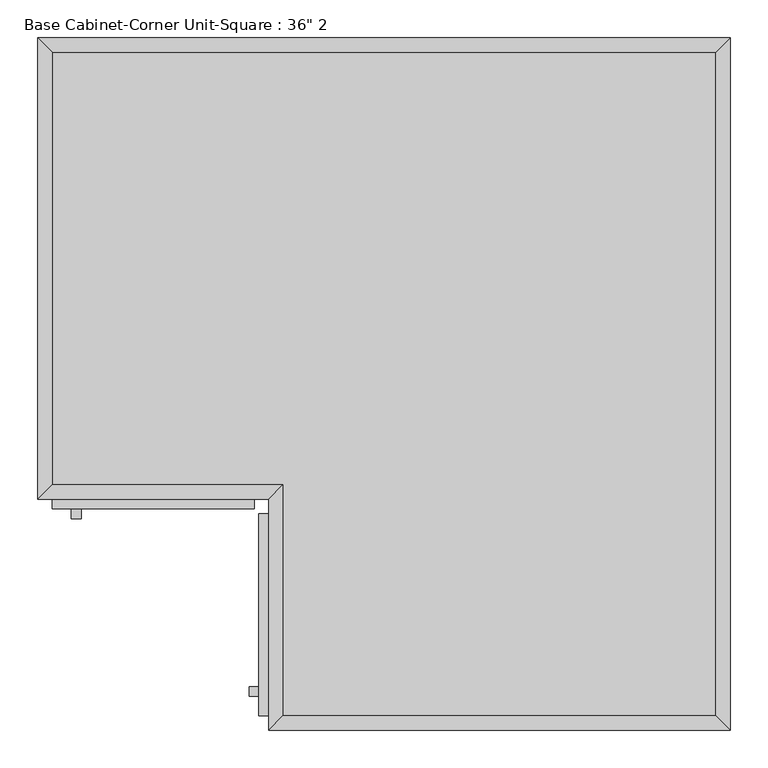
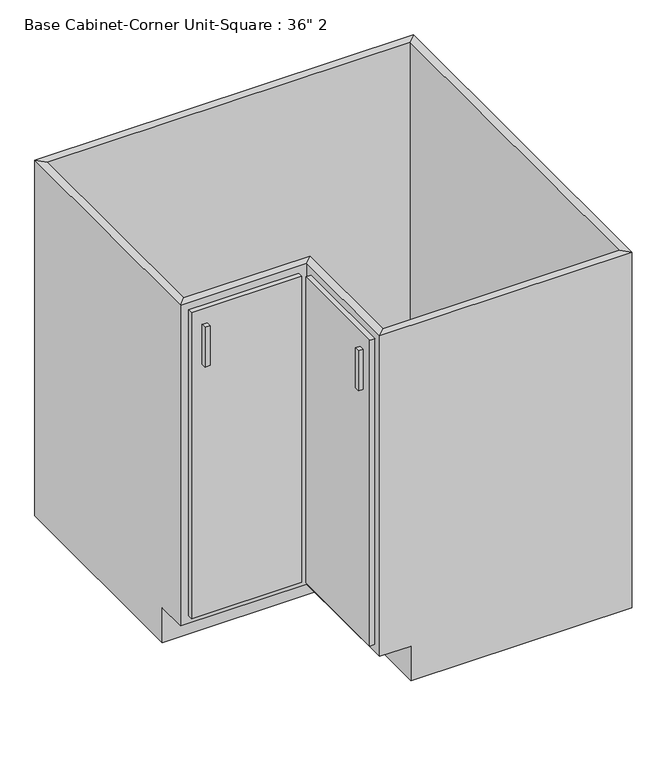
"""IFC4 building model written with IfcOpenShell, lengths in millimetres: furniture geometry."""

from ifc_helpers import new_model, si_unit, frame, origin, place, context, project, spatial, polyline, outline, extrude, faceted_brep, source, transform, mapped, element, save


def furniture_13b99e4d(model_context):
    return source(origin(), model_context, "Body", "SolidModel", [
        extrude(outline(polyline([(507.6877049, -19.05), (507.6877049, -895.35), (-63.8122951, -895.35), (-63.8122951, -590.55), (-368.6122951, -590.55), (-368.6122951, -19.05), (507.6877049, -19.05)])), frame((0.0, 0.0, 88.9), z_axis=(0.0, 0.0, 1.0), x_axis=(1.0, 0.0, 0.0)), (0.0, 0.0, 1.0), 19.05),
        extrude(outline(polyline([(-101.9122951, -622.3), (-368.6122951, -622.3), (-368.6122951, -609.6), (-101.9122951, -609.6), (-101.9122951, -622.3)])), frame((0.0, 0.0, 107.95), z_axis=(0.0, 0.0, 1.0), x_axis=(1.0, 0.0, 0.0)), (0.0, 0.0, 1.0), 781.05),
        extrude(outline(polyline([(-330.5122951, -635.0), (-343.2122951, -635.0), (-343.2122951, -622.3), (-330.5122951, -622.3), (-330.5122951, -635.0)])), frame((0.0, 0.0, 749.3), z_axis=(0.0, 0.0, 1.0), x_axis=(1.0, 0.0, 0.0)), (0.0, 0.0, 1.0), 101.6),
        extrude(outline(polyline([(-82.8622951, -628.65), (-82.8622951, -895.35), (-95.5622951, -895.35), (-95.5622951, -628.65), (-82.8622951, -628.65)])), frame((0.0, 0.0, 107.95), z_axis=(0.0, 0.0, 1.0), x_axis=(1.0, 0.0, 0.0)), (0.0, 0.0, 1.0), 781.05),
        extrude(outline(polyline([(-95.5622951, -857.25), (-95.5622951, -869.95), (-108.2622951, -869.95), (-108.2622951, -857.25), (-95.5622951, -857.25)])), frame((0.0, 0.0, 749.3), z_axis=(0.0, 0.0, 1.0), x_axis=(1.0, 0.0, 0.0)), (0.0, 0.0, 1.0), 101.6),
        faceted_brep([(-368.6122951, -533.4, 88.9), (-6.6622951, -533.4, 88.9), (-6.6622951, -895.35, 88.9), (507.6877049, -895.35, 88.9), (507.6877049, -19.05, 88.9), (-368.6122951, -19.05, 88.9), (526.7377049, 0.0, 0.0), (526.7377049, -914.4, 0.0), (-6.6622951, -914.4, 0.0), (-6.6622951, -533.4, 0.0), (-387.6622951, -533.4, 0.0), (-387.6622951, 0.0, 0.0), (-387.6622951, 0.0, 908.05), (526.7377049, 0.0, 908.05), (-387.6622951, -533.4, 88.9), (-387.6622951, -609.6, 88.9), (-387.6622951, -609.6, 908.05), (-6.6622951, -914.4, 88.9), (526.7377049, -914.4, 908.05), (-82.8622951, -914.4, 908.05), (-82.8622951, -914.4, 88.9), (507.6877049, -895.35, 908.05), (-63.8122951, -895.35, 88.9), (-63.8122951, -895.35, 908.05), (-63.8122951, -590.55, 88.9), (-63.8122951, -590.55, 908.05), (-82.8622951, -609.6, 908.05), (-82.8622951, -609.6, 88.9), (-368.6122951, -590.55, 88.9), (-368.6122951, -590.55, 908.05), (-368.6122951, -19.05, 908.05), (507.6877049, -19.05, 908.05)], [[[0, 1, 2, 3, 4, 5]], [[6, 7, 8, 9, 10, 11]], [[6, 11, 12, 13]], [[12, 11, 10, 14, 15, 16]], [[10, 9, 1, 0, 14]], [[9, 8, 17, 2, 1]], [[8, 7, 18, 19, 20, 17]], [[18, 7, 6, 13]], [[21, 3, 2, 22, 23]], [[21, 23, 19, 18]], [[20, 22, 2, 17]], [[23, 22, 24, 25]], [[19, 23, 25, 26]], [[20, 19, 26, 27]], [[22, 20, 27, 24]], [[25, 24, 28, 29]], [[26, 25, 29, 16]], [[27, 26, 16, 15]], [[24, 27, 15, 28]], [[29, 28, 0, 5, 30]], [[16, 29, 30, 12]], [[28, 15, 14, 0]], [[30, 5, 4, 31]], [[12, 30, 31, 13]], [[3, 21, 31, 4]], [[21, 18, 13, 31]]]),
    ])


if __name__ == "__main__":
    model = new_model("IFC4")
    model_context = context("Model", 3, world=origin())
    ifc_project = project(units=[si_unit("LENGTHUNIT", "METRE", prefix="MILLI")], contexts=[model_context])
    site = spatial("IfcSite", under=ifc_project)
    building = spatial("IfcBuilding", under=site)
    placement = place(None, origin())
    furniture_shape = furniture_13b99e4d(model_context)
    element("IfcFurniture", 1, ObjectType="Base Cabinet-Corner Unit-Square : 36\" 2", at=placement, inside=building, context=model_context, shape_type="MappedRepresentation", body=[
        mapped(furniture_shape, transform((0.0, 0.0, 0.0), x_axis=(1.0, 0.0, 0.0), y_axis=(0.0, 1.0, 0.0), z_axis=(0.0, 0.0, 1.0))),
    ])
    save(model, "model.ifc")

# Revit data of these elements
# Type "Base Cabinet-Corner Unit-Square : 36\" 2"
#   Assembly Code = "C1030410"
#   Depth = 2' - 0"
#   Height = 2' - 11 3/4"
#   Toe Depth = 0' - 3"
#   Toe Height = 0' - 3 1/2"
#   Width = 3' - 0"
#   Cabinet Material = Cabinets
#   Door/Drawer Material = Cabinets
#   Handle Material = Cabinets - Handles
#   Default Elevation = 0
# Element 1 (IfcFurniture, "Base Cabinet-Corner Unit-Square : 36\" 2")
#   Materials on its faces: "Cabinets", "Cabinets - Handles"
# Materials
#   "Cabinets": colour RGB 249 249 249, transparency 0
#   "Cabinets - Handles": colour RGB 57 57 57, transparency 0
